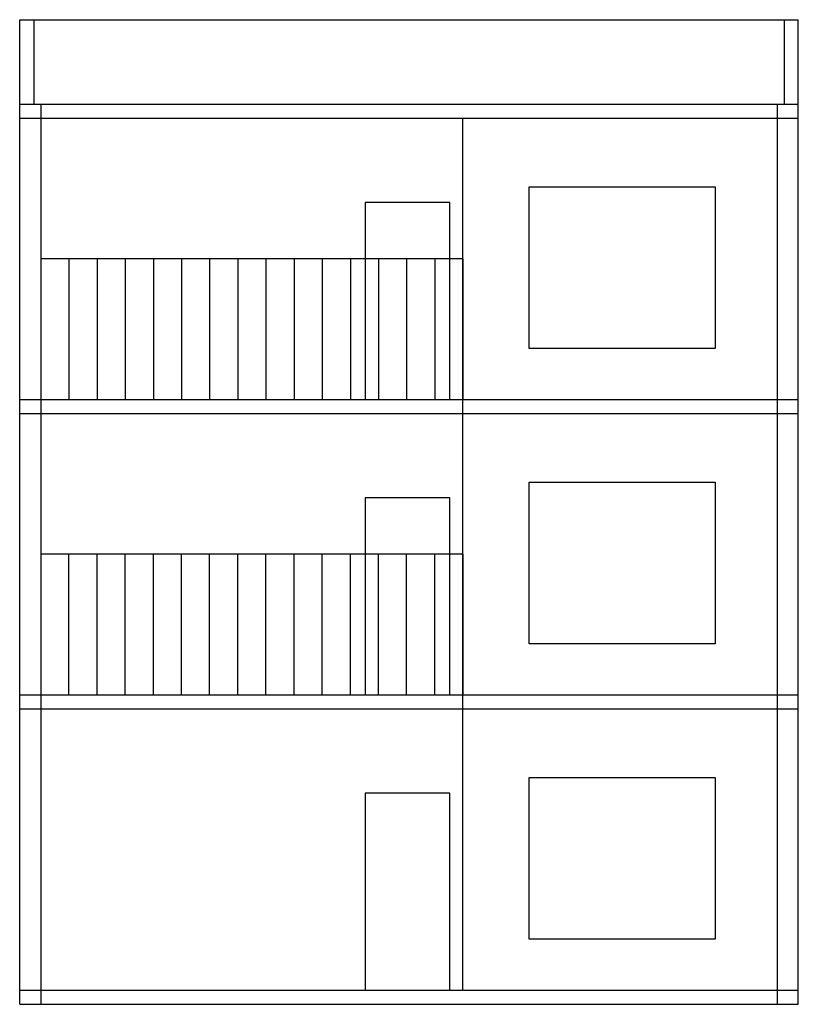
# Model space of a CAD drawing. Units: feet. Extents: x 993 to 3080, y -271 to 22562.
# Tile 1 of 4: x 1546 to 1878, y -244 to 176. Entities that reach past the tile are written whole.
import ezdxf

# ---------------------------------------------------------------- set-up
doc = ezdxf.new("R2010")
doc.units = ezdxf.units.FT
doc.layers.add('A-ELEV', color=7, linetype='Continuous', lineweight=25)

# ---------------------------------------------------------------- blocks, each defined once
blk = doc.blocks.new('DOOR-ELEV')
for p, q in [((36, 84), (0, 84)), ((0, 84), (0, 0)), ((36, 0), (36, 84))]:
    blk.add_line(p, q)

msp = doc.modelspace()

# ---------------------------------------------------------------- linework, layer by layer
at = {"layer": 'A-ELEV'}
for p, q in [((1545.91505, 13.57516), (1545.91505, 175.57516)), ((1545.91505, 175.57516), (1877.91505, 175.57516)), ((1545.91505, 175.57516), (1545.91505, 175.57516)), ((1551.91505, 175.57516), (1551.91505, 139.57516)), ((1871.91505, 175.57516), (1871.91505, 139.57516)), ((1877.91505, -244.42484), (1877.91505, 175.57516)), ((1545.91505, 139.57516), (1877.91505, 139.57516)), ((1554.91505, 139.57516), (1554.91505, -244.42484)), ((1868.91505, 139.57516), (1868.91505, -244.42484)), ((1545.91505, 133.57516), (1877.91505, 133.57516)), ((1734.91505, -238.42484), (1734.91505, 133.57516)), ((1734.91505, 73.57516), (1554.91505, 73.57516)), ((1566.91505, 73.57516), (1566.91505, 13.57516)), ((1578.91505, 73.57516), (1578.91505, 13.57516)), ((1590.91505, 73.57516), (1590.91505, 13.57516)), ((1602.91505, 73.57516), (1602.91505, 13.57516)), ((1614.91505, 73.57516), (1614.91505, 13.57516)), ((1626.91505, 73.57516), (1626.91505, 13.57516)), ((1638.91505, 73.57516), (1638.91505, 13.57516)), ((1650.91505, 73.57516), (1650.91505, 13.57516)), ((1662.91505, 73.57516), (1662.91505, 13.57516)), ((1674.91505, 73.57516), (1674.91505, 13.57516)), ((1686.91505, 73.57516), (1686.91505, 13.57516)), ((1698.91505, 73.57516), (1698.91505, 13.57516)), ((1710.91505, 73.57516), (1710.91505, 13.57516)), ((1722.91505, 73.57516), (1722.91505, 13.57516)), ((1734.91505, 73.57516), (1734.91505, 13.57516)), ((1545.91505, 7.57516), (1545.91505, 13.57516)), ((1545.91505, 13.57516), (1877.91505, 13.57516)), ((1545.91505, -112.42484), (1545.91505, 7.57516)), ((1545.91505, 7.57516), (1877.91505, 7.57516)), ((1734.91505, -52.42484), (1554.91505, -52.42484)), ((1566.91505, -112.42484), (1566.91505, -52.42484)), ((1578.91505, -112.42484), (1578.91505, -52.42484)), ((1590.91505, -112.42484), (1590.91505, -52.42484)), ((1602.91505, -112.42484), (1602.91505, -52.42484)), ((1614.91505, -112.42484), (1614.91505, -52.42484)), ((1626.91505, -112.42484), (1626.91505, -52.42484)), ((1638.91505, -112.42484), (1638.91505, -52.42484)), ((1650.91505, -112.42484), (1650.91505, -52.42484)), ((1662.91505, -112.42484), (1662.91505, -52.42484)), ((1674.91505, -112.42484), (1674.91505, -52.42484)), ((1686.91505, -112.42484), (1686.91505, -52.42484)), ((1698.91505, -112.42484), (1698.91505, -52.42484)), ((1710.91505, -112.42484), (1710.91505, -52.42484)), ((1722.91505, -112.42484), (1722.91505, -52.42484)), ((1734.91505, -112.42484), (1734.91505, -52.42484)), ((1734.91505, -52.42484), (1734.91505, -112.42484)), ((1545.91505, -118.42484), (1545.91505, -112.42484)), ((1545.91505, -112.42484), (1877.91505, -112.42484)), ((1545.91505, -244.42484), (1545.91505, -118.42484)), ((1545.91505, -118.42484), (1877.91505, -118.42484)), ((1545.91505, -238.42484), (1877.91505, -238.42484)), ((1545.91505, -244.42484), (1877.91505, -244.42484))]:
    msp.add_line(p, q, dxfattribs=at)
for points in [[(1763.19169, 104.34033), (1842.48854, 104.34033), (1842.48854, 35.36473), (1763.19169, 35.36473)], [(1763.19169, -21.65967), (1842.48854, -21.65967), (1842.48854, -90.63527), (1763.19169, -90.63527)], [(1763.19169, -147.65967), (1842.48854, -147.65967), (1842.48854, -216.63527), (1763.19169, -216.63527)]]:
    msp.add_lwpolyline(points, close=True, dxfattribs=at)

# ---------------------------------------------------------------- block references
for p in [(1693.27, 13.575), (1693.27, -112.425), (1693.27, -238.425)]:
    msp.add_blockref('DOOR-ELEV', p, dxfattribs=at)

doc.saveas('drawing.dxf')
